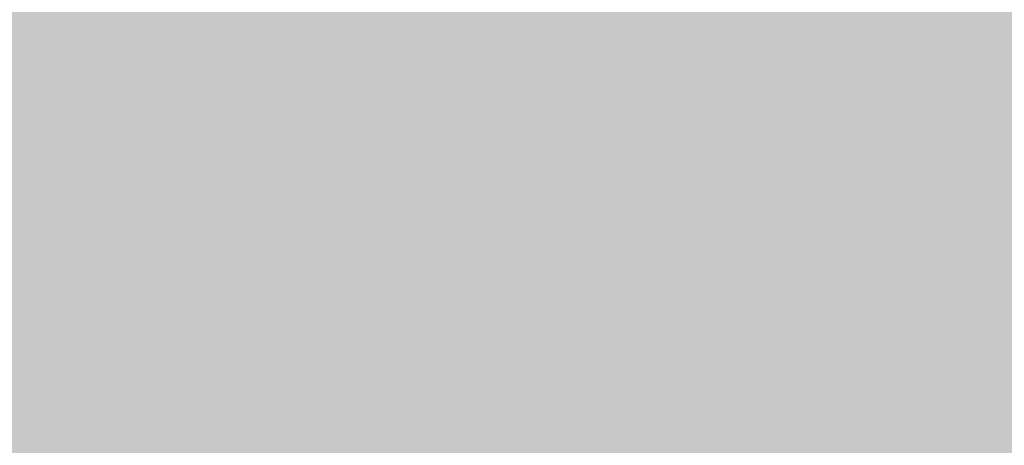
# Model space of a CAD drawing. Units: millimetres. Extents: x -22994 to 29398, y -19990 to 20176.
# Tile 74 of 135: x 226.355 to 227.437, y 83.796 to 84.264. Entities that reach past the tile are written whole.
import ezdxf
from ezdxf import colors
from ezdxf.entities.mleader import LeaderData, LeaderLine
from ezdxf.math import Vec2, Vec3

# ---------------------------------------------------------------- set-up
doc = ezdxf.new("R2010")
doc.units = ezdxf.units.MM
doc.header["$MEASUREMENT"] = 0
for name, color, linetype, lineweight in [('M-ANNO-TEXT', 7, 'Continuous', 25), ('M-DIMS', 2, 'Continuous', 18), ('M-EQPM-PATT', 7, 'Continuous', 18)]:
    doc.layers.add(name, color=color, linetype=linetype, lineweight=lineweight)
doc.styles.get("Standard").update_dxf_attribs({"font": 'arial.ttf'})
doc.dimstyles.get("Standard").update_dxf_attribs({"dimtxt": 0.18, "dimasz": 10000, "dimexe": 0.18, "dimexo": 0.0625, "dimgap": 0.09, "dimtad": 0, "dimtih": 1, "dimtoh": 1, "dimdec": 0, "dimzin": 0, "dimdsep": 46, "dimtxsty": 'Standard', "dimcen": 0.09, "dimadec": 0, "dimazin": 0, "dimtfac": 1, "dimtdec": 0, "dimtofl": 0, "dimtmove": 0, "dimatfit": 3, "dimfxl": 1, "dimtolj": 1, "dimtzin": 0, "dimlwd": 30, "dimarcsym": 0})

# ---------------------------------------------------------------- blocks, each defined once
blk = doc.blocks.new('*D2')
at = {"layer": 'Defpoints', "color": 0, "transparency": 16777216}
for p in [(6.6773, 10.2713), (290.852, 10.2713), (290.852, -5.0787)]:
    blk.add_point(p, dxfattribs=at)
at = {"layer": 'M-DIMS', "color": 0, "lineweight": -2, "transparency": 16777216}
for p, q in [((6.6773, 10.2088), (6.6773, -5.2587)), ((290.852, 10.2088), (290.852, -5.2587))]:
    blk.add_line(p, q, dxfattribs=at)
at = {"layer": 'M-DIMS', "color": 0, "lineweight": 30, "transparency": 16777216}
for p, q in [((-9993.3227, -5.0787), (-19993.3227, -5.0787)), ((10290.852, -5.0787), (20290.852, -5.0787))]:
    blk.add_line(p, q, dxfattribs=at)
at = {"layer": 'M-DIMS', "color": 0, "transparency": 16777216}
for points in [[(-9993.3227, 1661.5879), (-9993.3227, -1671.7454), (6.6773, -5.0787)], [(10290.852, 1661.5879), (10290.852, -1671.7454), (290.852, -5.0787)]]:
    blk.add_solid(points, dxfattribs=at)
at = {"layer": 'M-DIMS', "color": 0, "transparency": 16777216, "insert": (148.7647, -5.0787), "char_height": 0.18, "attachment_point": 5}
blk.add_mtext('\\A1;284.2', dxfattribs=at)
blk = doc.blocks.new('*D3')
at = {"layer": 'Defpoints', "color": 0, "transparency": 16777216}
for p in [(110.2647, 204.1654), (110.2647, 176.3662), (95.8327, 127.967)]:
    blk.add_point(p, dxfattribs=at)
at = {"layer": 'M-DIMS', "color": 0, "lineweight": -2, "transparency": 16777216}
for p, q in [((95.8327, 128.0295), (95.8327, 204.3454)), ((110.2647, 176.4287), (110.2647, 204.3454))]:
    blk.add_line(p, q, dxfattribs=at)
at = {"layer": 'M-DIMS', "color": 0, "lineweight": 30, "transparency": 16777216}
for p, q in [((-9904.1673, 204.1654), (-19904.1673, 204.1654)), ((10110.2647, 204.1654), (20110.2647, 204.1654))]:
    blk.add_line(p, q, dxfattribs=at)
at = {"layer": 'M-DIMS', "color": 0, "transparency": 16777216}
for points in [[(-9904.1673, 1870.8321), (-9904.1673, -1462.5013), (95.8327, 204.1654)], [(10110.2647, 1870.8321), (10110.2647, -1462.5013), (110.2647, 204.1654)]]:
    blk.add_solid(points, dxfattribs=at)
at = {"layer": 'M-DIMS', "color": 0, "transparency": 16777216, "insert": (103.0487, 204.1654), "char_height": 0.18, "attachment_point": 5}
blk.add_mtext('\\A1;14.432', dxfattribs=at)
blk = doc.blocks.new('*D4')
at = {"layer": 'Defpoints', "color": 0, "transparency": 16777216}
for p in [(116.2647, 204.1654), (110.2647, 176.3662), (116.2647, 176.3662)]:
    blk.add_point(p, dxfattribs=at)
at = {"layer": 'M-DIMS', "color": 0, "lineweight": -2, "transparency": 16777216}
for p, q in [((110.2647, 176.4287), (110.2647, 204.3454)), ((116.2647, 176.4287), (116.2647, 204.3454))]:
    blk.add_line(p, q, dxfattribs=at)
at = {"layer": 'M-DIMS', "color": 0, "lineweight": 30, "transparency": 16777216}
for p, q in [((-9889.7353, 204.1654), (-19889.7353, 204.1654)), ((10116.2647, 204.1654), (20116.2647, 204.1654))]:
    blk.add_line(p, q, dxfattribs=at)
at = {"layer": 'M-DIMS', "color": 0, "transparency": 16777216}
for points in [[(-9889.7353, 1870.8321), (-9889.7353, -1462.5013), (110.2647, 204.1654)], [(10116.2647, 1870.8321), (10116.2647, -1462.5013), (116.2647, 204.1654)]]:
    blk.add_solid(points, dxfattribs=at)
at = {"layer": 'M-DIMS', "color": 0, "transparency": 16777216, "insert": (113.2647, 204.1654), "char_height": 0.18, "attachment_point": 5}
blk.add_mtext('\\A1;6', dxfattribs=at)
blk = doc.blocks.new('*D5')
at = {"layer": 'Defpoints', "color": 0, "transparency": 16777216}
for p in [(181.2647, 204.1654), (116.2647, 176.3662), (181.2647, 176.3662)]:
    blk.add_point(p, dxfattribs=at)
at = {"layer": 'M-DIMS', "color": 0, "lineweight": -2, "transparency": 16777216}
for p, q in [((116.2647, 176.4287), (116.2647, 204.3454)), ((181.2647, 176.4287), (181.2647, 204.3454))]:
    blk.add_line(p, q, dxfattribs=at)
at = {"layer": 'M-DIMS', "color": 0, "lineweight": 30, "transparency": 16777216}
for p, q in [((-9883.7353, 204.1654), (-19883.7353, 204.1654)), ((10181.2647, 204.1654), (20181.2647, 204.1654))]:
    blk.add_line(p, q, dxfattribs=at)
at = {"layer": 'M-DIMS', "color": 0, "transparency": 16777216}
for points in [[(-9883.7353, 1870.8321), (-9883.7353, -1462.5013), (116.2647, 204.1654)], [(10181.2647, 1870.8321), (10181.2647, -1462.5013), (181.2647, 204.1654)]]:
    blk.add_solid(points, dxfattribs=at)
at = {"layer": 'M-DIMS', "color": 0, "transparency": 16777216, "insert": (148.7647, 204.1654), "char_height": 0.18, "attachment_point": 5}
blk.add_mtext('\\A1;65', dxfattribs=at)
blk = doc.blocks.new('*D6')
at = {"layer": 'Defpoints', "color": 0, "transparency": 16777216}
for p in [(187.2647, 204.1654), (181.2647, 176.3662), (187.2647, 176.3662)]:
    blk.add_point(p, dxfattribs=at)
at = {"layer": 'M-DIMS', "color": 0, "lineweight": -2, "transparency": 16777216}
for p, q in [((181.2647, 176.4287), (181.2647, 204.3454)), ((187.2647, 176.4287), (187.2647, 204.3454))]:
    blk.add_line(p, q, dxfattribs=at)
at = {"layer": 'M-DIMS', "color": 0, "lineweight": 30, "transparency": 16777216}
for p, q in [((-9818.7353, 204.1654), (-19818.7353, 204.1654)), ((10187.2647, 204.1654), (20187.2647, 204.1654))]:
    blk.add_line(p, q, dxfattribs=at)
at = {"layer": 'M-DIMS', "color": 0, "transparency": 16777216}
for points in [[(-9818.7353, 1870.8321), (-9818.7353, -1462.5013), (181.2647, 204.1654)], [(10187.2647, 1870.8321), (10187.2647, -1462.5013), (187.2647, 204.1654)]]:
    blk.add_solid(points, dxfattribs=at)
at = {"layer": 'M-DIMS', "color": 0, "transparency": 16777216, "insert": (184.2647, 204.1654), "char_height": 0.18, "attachment_point": 5}
blk.add_mtext('\\A1;6', dxfattribs=at)
blk = doc.blocks.new('*D7')
at = {"layer": 'Defpoints', "color": 0, "transparency": 16777216}
for p in [(201.6967, 204.1654), (187.2647, 176.3662), (201.6967, 127.967)]:
    blk.add_point(p, dxfattribs=at)
at = {"layer": 'M-DIMS', "color": 0, "lineweight": -2, "transparency": 16777216}
for p, q in [((187.2647, 176.4287), (187.2647, 204.3454)), ((201.6967, 128.0295), (201.6967, 204.3454))]:
    blk.add_line(p, q, dxfattribs=at)
at = {"layer": 'M-DIMS', "color": 0, "lineweight": 30, "transparency": 16777216}
for p, q in [((-9812.7353, 204.1654), (-19812.7353, 204.1654)), ((10201.6967, 204.1654), (20201.6967, 204.1654))]:
    blk.add_line(p, q, dxfattribs=at)
at = {"layer": 'M-DIMS', "color": 0, "transparency": 16777216}
for points in [[(-9812.7353, 1870.8321), (-9812.7353, -1462.5013), (187.2647, 204.1654)], [(10201.6967, 1870.8321), (10201.6967, -1462.5013), (201.6967, 204.1654)]]:
    blk.add_solid(points, dxfattribs=at)
at = {"layer": 'M-DIMS', "color": 0, "transparency": 16777216, "insert": (194.4807, 204.1654), "char_height": 0.18, "attachment_point": 5}
blk.add_mtext('\\A1;14.432', dxfattribs=at)
blk = doc.blocks.new('*D8')
at = {"layer": 'Defpoints', "color": 0, "transparency": 16777216}
for p in [(227.6485, 204.1654), (227.6485, 146.7296), (201.6967, 127.967)]:
    blk.add_point(p, dxfattribs=at)
at = {"layer": 'M-DIMS', "color": 0, "lineweight": -2, "transparency": 16777216}
for p, q in [((201.6967, 128.0295), (201.6967, 204.3454)), ((227.6485, 146.7921), (227.6485, 204.3454))]:
    blk.add_line(p, q, dxfattribs=at)
at = {"layer": 'M-DIMS', "color": 0, "lineweight": 30, "transparency": 16777216}
for p, q in [((-9798.3033, 204.1654), (-19798.3033, 204.1654)), ((10227.6485, 204.1654), (20227.6485, 204.1654))]:
    blk.add_line(p, q, dxfattribs=at)
at = {"layer": 'M-DIMS', "color": 0, "transparency": 16777216}
for points in [[(-9798.3033, 1870.8321), (-9798.3033, -1462.5013), (201.6967, 204.1654)], [(10227.6485, 1870.8321), (10227.6485, -1462.5013), (227.6485, 204.1654)]]:
    blk.add_solid(points, dxfattribs=at)
at = {"layer": 'M-DIMS', "color": 0, "transparency": 16777216, "insert": (214.6726, 204.1654), "char_height": 0.18, "attachment_point": 5}
blk.add_mtext('\\A1;25.95', dxfattribs=at)
blk = doc.blocks.new('*D9')
at = {"layer": 'Defpoints', "color": 0, "transparency": 16777216}
for p in [(187.2647, 176.3662), (306.202, 176.3662), (290.852, 10.2713)]:
    blk.add_point(p, dxfattribs=at)
at = {"layer": 'M-DIMS', "color": 0, "lineweight": 30, "transparency": 16777216}
for p, q in [((306.202, 10176.3662), (306.202, 20176.3662)), ((306.202, -9989.7287), (306.202, -19989.7287))]:
    blk.add_line(p, q, dxfattribs=at)
at = {"layer": 'M-DIMS', "color": 0, "lineweight": -2, "transparency": 16777216}
for p, q in [((187.3272, 176.3662), (306.382, 176.3662)), ((290.9145, 10.2713), (306.382, 10.2713))]:
    blk.add_line(p, q, dxfattribs=at)
at = {"layer": 'M-DIMS', "color": 0, "transparency": 16777216}
for points in [[(-1360.4646, 10176.3662), (1972.8687, 10176.3662), (306.202, 176.3662)], [(-1360.4646, -9989.7287), (1972.8687, -9989.7287), (306.202, 10.2713)]]:
    blk.add_solid(points, dxfattribs=at)
at = {"layer": 'M-DIMS', "color": 0, "transparency": 16777216, "insert": (306.202, 93.3187), "char_height": 0.18, "attachment_point": 5}
blk.add_mtext('\\A1;166.1', dxfattribs=at)
blk = doc.blocks.new('*D10')
at = {"layer": 'Defpoints', "color": 0, "transparency": 16777216}
for p in [(125.6498, 136.0713), (133.3459, 136.0713), (133.3459, -5.0787)]:
    blk.add_point(p, dxfattribs=at)
at = {"layer": 'M-DIMS', "color": 0, "lineweight": -2, "transparency": 16777216}
for p, q in [((125.6498, 136.0088), (125.6498, -5.2587)), ((133.3459, 136.0088), (133.3459, -5.2587))]:
    blk.add_line(p, q, dxfattribs=at)
at = {"layer": 'M-DIMS', "color": 0, "lineweight": 30, "transparency": 16777216}
for p, q in [((-9874.3502, -5.0787), (-19874.3502, -5.0787)), ((10133.3459, -5.0787), (20133.3459, -5.0787))]:
    blk.add_line(p, q, dxfattribs=at)
at = {"layer": 'M-DIMS', "color": 0, "transparency": 16777216}
for points in [[(-9874.3502, 1661.5879), (-9874.3502, -1671.7454), (125.6498, -5.0787)], [(10133.3459, 1661.5879), (10133.3459, -1671.7454), (133.3459, -5.0787)]]:
    blk.add_solid(points, dxfattribs=at)
at = {"layer": 'M-DIMS', "color": 0, "transparency": 16777216, "insert": (129.4978, -5.0787), "char_height": 0.18, "attachment_point": 5}
blk.add_mtext('\\A1;7.696', dxfattribs=at)
blk = doc.blocks.new('*D11')
at = {"layer": 'Defpoints', "color": 0, "transparency": 16777216}
for p in [(133.3459, 136.0713), (135.6498, 136.0713), (135.6498, -5.0787)]:
    blk.add_point(p, dxfattribs=at)
at = {"layer": 'M-DIMS', "color": 0, "lineweight": -2, "transparency": 16777216}
for p, q in [((133.3459, 136.0088), (133.3459, -5.2587)), ((135.6498, 136.0088), (135.6498, -5.2587))]:
    blk.add_line(p, q, dxfattribs=at)
at = {"layer": 'M-DIMS', "color": 0, "lineweight": 30, "transparency": 16777216}
for p, q in [((-9866.6541, -5.0787), (-19866.6541, -5.0787)), ((10135.6498, -5.0787), (20135.6498, -5.0787))]:
    blk.add_line(p, q, dxfattribs=at)
at = {"layer": 'M-DIMS', "color": 0, "transparency": 16777216}
for points in [[(-9866.6541, 1661.5879), (-9866.6541, -1671.7454), (133.3459, -5.0787)], [(10135.6498, 1661.5879), (10135.6498, -1671.7454), (135.6498, -5.0787)]]:
    blk.add_solid(points, dxfattribs=at)
at = {"layer": 'M-DIMS', "color": 0, "transparency": 16777216, "insert": (134.4978, -5.0787), "char_height": 0.18, "attachment_point": 5}
blk.add_mtext('\\A1;2.304', dxfattribs=at)
blk = doc.blocks.new('*D12')
at = {"layer": 'Defpoints', "color": 0, "transparency": 16777216}
for p in [(135.6498, 136.0713), (145.6498, 136.0713), (145.6498, -5.0787)]:
    blk.add_point(p, dxfattribs=at)
at = {"layer": 'M-DIMS', "color": 0, "lineweight": -2, "transparency": 16777216}
for p, q in [((135.6498, 136.0088), (135.6498, -5.2587)), ((145.6498, 136.0088), (145.6498, -5.2587))]:
    blk.add_line(p, q, dxfattribs=at)
at = {"layer": 'M-DIMS', "color": 0, "lineweight": 30, "transparency": 16777216}
for p, q in [((-9864.3502, -5.0787), (-19864.3502, -5.0787)), ((10145.6498, -5.0787), (20145.6498, -5.0787))]:
    blk.add_line(p, q, dxfattribs=at)
at = {"layer": 'M-DIMS', "color": 0, "transparency": 16777216}
for points in [[(-9864.3502, 1661.5879), (-9864.3502, -1671.7454), (135.6498, -5.0787)], [(10145.6498, 1661.5879), (10145.6498, -1671.7454), (145.6498, -5.0787)]]:
    blk.add_solid(points, dxfattribs=at)
at = {"layer": 'M-DIMS', "color": 0, "transparency": 16777216, "insert": (140.6498, -5.0787), "char_height": 0.18, "attachment_point": 5}
blk.add_mtext('\\A1;10', dxfattribs=at)
blk = doc.blocks.new('*D13')
at = {"layer": 'Defpoints', "color": 0, "transparency": 16777216}
for p in [(145.6498, 136.0713), (155.6498, 136.0713), (155.6498, -5.0787)]:
    blk.add_point(p, dxfattribs=at)
at = {"layer": 'M-DIMS', "color": 0, "lineweight": -2, "transparency": 16777216}
for p, q in [((145.6498, 136.0088), (145.6498, -5.2587)), ((155.6498, 136.0088), (155.6498, -5.2587))]:
    blk.add_line(p, q, dxfattribs=at)
at = {"layer": 'M-DIMS', "color": 0, "lineweight": 30, "transparency": 16777216}
for p, q in [((-9854.3502, -5.0787), (-19854.3502, -5.0787)), ((10155.6498, -5.0787), (20155.6498, -5.0787))]:
    blk.add_line(p, q, dxfattribs=at)
at = {"layer": 'M-DIMS', "color": 0, "transparency": 16777216}
for points in [[(-9854.3502, 1661.5879), (-9854.3502, -1671.7454), (145.6498, -5.0787)], [(10155.6498, 1661.5879), (10155.6498, -1671.7454), (155.6498, -5.0787)]]:
    blk.add_solid(points, dxfattribs=at)
at = {"layer": 'M-DIMS', "color": 0, "transparency": 16777216, "insert": (150.6498, -5.0787), "char_height": 0.18, "attachment_point": 5}
blk.add_mtext('\\A1;10', dxfattribs=at)
blk = doc.blocks.new('*D14')
at = {"layer": 'Defpoints', "color": 0, "transparency": 16777216}
for p in [(155.6498, 136.0713), (165.6498, 136.0713), (165.6498, -5.0787)]:
    blk.add_point(p, dxfattribs=at)
at = {"layer": 'M-DIMS', "color": 0, "lineweight": -2, "transparency": 16777216}
for p, q in [((155.6498, 136.0088), (155.6498, -5.2587)), ((165.6498, 136.0088), (165.6498, -5.2587))]:
    blk.add_line(p, q, dxfattribs=at)
at = {"layer": 'M-DIMS', "color": 0, "lineweight": 30, "transparency": 16777216}
for p, q in [((-9844.3502, -5.0787), (-19844.3502, -5.0787)), ((10165.6498, -5.0787), (20165.6498, -5.0787))]:
    blk.add_line(p, q, dxfattribs=at)
at = {"layer": 'M-DIMS', "color": 0, "transparency": 16777216}
for points in [[(-9844.3502, 1661.5879), (-9844.3502, -1671.7454), (155.6498, -5.0787)], [(10165.6498, 1661.5879), (10165.6498, -1671.7454), (165.6498, -5.0787)]]:
    blk.add_solid(points, dxfattribs=at)
at = {"layer": 'M-DIMS', "color": 0, "transparency": 16777216, "insert": (160.6498, -5.0787), "char_height": 0.18, "attachment_point": 5}
blk.add_mtext('\\A1;10', dxfattribs=at)
blk = doc.blocks.new('*D15')
at = {"layer": 'Defpoints', "color": 0, "transparency": 16777216}
for p in [(173.3459, 154.788), (173.3459, 136.0713), (306.202, 136.0713)]:
    blk.add_point(p, dxfattribs=at)
at = {"layer": 'M-DIMS', "color": 0, "lineweight": 30, "transparency": 16777216}
for p, q in [((306.202, 10154.788), (306.202, 20154.788)), ((306.202, -9863.9287), (306.202, -19863.9287))]:
    blk.add_line(p, q, dxfattribs=at)
at = {"layer": 'M-DIMS', "color": 0, "lineweight": -2, "transparency": 16777216}
for p, q in [((173.4084, 154.788), (306.382, 154.788)), ((173.4084, 136.0713), (306.382, 136.0713))]:
    blk.add_line(p, q, dxfattribs=at)
at = {"layer": 'M-DIMS', "color": 0, "transparency": 16777216}
for points in [[(-1360.4646, 10154.788), (1972.8687, 10154.788), (306.202, 154.788)], [(-1360.4646, -9863.9287), (1972.8687, -9863.9287), (306.202, 136.0713)]]:
    blk.add_solid(points, dxfattribs=at)
at = {"layer": 'M-DIMS', "color": 0, "transparency": 16777216, "insert": (306.202, 145.4297), "char_height": 0.18, "attachment_point": 5}
blk.add_mtext('\\A1;18.717', dxfattribs=at)
blk = doc.blocks.new('*D16')
at = {"layer": 'Defpoints', "color": 0, "transparency": 16777216}
for p in [(120.1702, 204.1654), (110.4658, 48.0349), (120.1702, 48.0349)]:
    blk.add_point(p, dxfattribs=at)
at = {"layer": 'M-DIMS', "color": 0, "lineweight": -2, "transparency": 16777216}
for p, q in [((110.4658, 48.0974), (110.4658, 204.3454)), ((120.1702, 48.0974), (120.1702, 204.3454))]:
    blk.add_line(p, q, dxfattribs=at)
at = {"layer": 'M-DIMS', "color": 0, "lineweight": 30, "transparency": 16777216}
for p, q in [((-9889.5342, 204.1654), (-19889.5342, 204.1654)), ((10120.1702, 204.1654), (20120.1702, 204.1654))]:
    blk.add_line(p, q, dxfattribs=at)
at = {"layer": 'M-DIMS', "color": 0, "transparency": 16777216}
for points in [[(-9889.5342, 1870.8321), (-9889.5342, -1462.5013), (110.4658, 204.1654)], [(10120.1702, 1870.8321), (10120.1702, -1462.5013), (120.1702, 204.1654)]]:
    blk.add_solid(points, dxfattribs=at)
at = {"layer": 'M-DIMS', "color": 0, "transparency": 16777216, "insert": (115.318, 204.1654), "char_height": 0.18, "attachment_point": 5}
blk.add_mtext('\\A1;9.704', dxfattribs=at)
blk = doc.blocks.new('*D17')
at = {"layer": 'Defpoints', "color": 0, "transparency": 16777216}
for p in [(126.1702, 204.1654), (120.1702, 48.0349), (126.1702, 48.0349)]:
    blk.add_point(p, dxfattribs=at)
at = {"layer": 'M-DIMS', "color": 0, "lineweight": -2, "transparency": 16777216}
for p, q in [((120.1702, 48.0974), (120.1702, 204.3454)), ((126.1702, 48.0974), (126.1702, 204.3454))]:
    blk.add_line(p, q, dxfattribs=at)
at = {"layer": 'M-DIMS', "color": 0, "lineweight": 30, "transparency": 16777216}
for p, q in [((-9879.8298, 204.1654), (-19879.8298, 204.1654)), ((10126.1702, 204.1654), (20126.1702, 204.1654))]:
    blk.add_line(p, q, dxfattribs=at)
at = {"layer": 'M-DIMS', "color": 0, "transparency": 16777216}
for points in [[(-9879.8298, 1870.8321), (-9879.8298, -1462.5013), (120.1702, 204.1654)], [(10126.1702, 1870.8321), (10126.1702, -1462.5013), (126.1702, 204.1654)]]:
    blk.add_solid(points, dxfattribs=at)
at = {"layer": 'M-DIMS', "color": 0, "transparency": 16777216, "insert": (123.1702, 204.1654), "char_height": 0.18, "attachment_point": 5}
blk.add_mtext('\\A1;6', dxfattribs=at)
blk = doc.blocks.new('*D18')
at = {"layer": 'Defpoints', "color": 0, "transparency": 16777216}
for p in [(132.1702, 204.1654), (126.1702, 48.0349), (132.1702, 48.0349)]:
    blk.add_point(p, dxfattribs=at)
at = {"layer": 'M-DIMS', "color": 0, "lineweight": -2, "transparency": 16777216}
for p, q in [((126.1702, 48.0974), (126.1702, 204.3454)), ((132.1702, 48.0974), (132.1702, 204.3454))]:
    blk.add_line(p, q, dxfattribs=at)
at = {"layer": 'M-DIMS', "color": 0, "lineweight": 30, "transparency": 16777216}
for p, q in [((-9873.8298, 204.1654), (-19873.8298, 204.1654)), ((10132.1702, 204.1654), (20132.1702, 204.1654))]:
    blk.add_line(p, q, dxfattribs=at)
at = {"layer": 'M-DIMS', "color": 0, "transparency": 16777216}
for points in [[(-9873.8298, 1870.8321), (-9873.8298, -1462.5013), (126.1702, 204.1654)], [(10132.1702, 1870.8321), (10132.1702, -1462.5013), (132.1702, 204.1654)]]:
    blk.add_solid(points, dxfattribs=at)
at = {"layer": 'M-DIMS', "color": 0, "transparency": 16777216, "insert": (129.1702, 204.1654), "char_height": 0.18, "attachment_point": 5}
blk.add_mtext('\\A1;6', dxfattribs=at)
blk = doc.blocks.new('*D19')
at = {"layer": 'Defpoints', "color": 0, "transparency": 16777216}
for p in [(138.1702, 204.1654), (132.1702, 48.0349), (138.1702, 48.0349)]:
    blk.add_point(p, dxfattribs=at)
at = {"layer": 'M-DIMS', "color": 0, "lineweight": -2, "transparency": 16777216}
for p, q in [((132.1702, 48.0974), (132.1702, 204.3454)), ((138.1702, 48.0974), (138.1702, 204.3454))]:
    blk.add_line(p, q, dxfattribs=at)
at = {"layer": 'M-DIMS', "color": 0, "lineweight": 30, "transparency": 16777216}
for p, q in [((-9867.8298, 204.1654), (-19867.8298, 204.1654)), ((10138.1702, 204.1654), (20138.1702, 204.1654))]:
    blk.add_line(p, q, dxfattribs=at)
at = {"layer": 'M-DIMS', "color": 0, "transparency": 16777216}
for points in [[(-9867.8298, 1870.8321), (-9867.8298, -1462.5013), (132.1702, 204.1654)], [(10138.1702, 1870.8321), (10138.1702, -1462.5013), (138.1702, 204.1654)]]:
    blk.add_solid(points, dxfattribs=at)
at = {"layer": 'M-DIMS', "color": 0, "transparency": 16777216, "insert": (135.1702, 204.1654), "char_height": 0.18, "attachment_point": 5}
blk.add_mtext('\\A1;6', dxfattribs=at)
blk = doc.blocks.new('*D20')
at = {"layer": 'Defpoints', "color": 0, "transparency": 16777216}
for p in [(144.1702, 204.1654), (138.1702, 48.0349), (144.1702, 48.0349)]:
    blk.add_point(p, dxfattribs=at)
at = {"layer": 'M-DIMS', "color": 0, "lineweight": -2, "transparency": 16777216}
for p, q in [((138.1702, 48.0974), (138.1702, 204.3454)), ((144.1702, 48.0974), (144.1702, 204.3454))]:
    blk.add_line(p, q, dxfattribs=at)
at = {"layer": 'M-DIMS', "color": 0, "lineweight": 30, "transparency": 16777216}
for p, q in [((-9861.8298, 204.1654), (-19861.8298, 204.1654)), ((10144.1702, 204.1654), (20144.1702, 204.1654))]:
    blk.add_line(p, q, dxfattribs=at)
at = {"layer": 'M-DIMS', "color": 0, "transparency": 16777216}
for points in [[(-9861.8298, 1870.8321), (-9861.8298, -1462.5013), (138.1702, 204.1654)], [(10144.1702, 1870.8321), (10144.1702, -1462.5013), (144.1702, 204.1654)]]:
    blk.add_solid(points, dxfattribs=at)
at = {"layer": 'M-DIMS', "color": 0, "transparency": 16777216, "insert": (141.1702, 204.1654), "char_height": 0.18, "attachment_point": 5}
blk.add_mtext('\\A1;6', dxfattribs=at)
blk = doc.blocks.new('*D21')
at = {"layer": 'Defpoints', "color": 0, "transparency": 16777216}
for p in [(149.1157, 204.1654), (144.1702, 48.0349), (149.1157, 48.0349)]:
    blk.add_point(p, dxfattribs=at)
at = {"layer": 'M-DIMS', "color": 0, "lineweight": -2, "transparency": 16777216}
for p, q in [((144.1702, 48.0974), (144.1702, 204.3454)), ((149.1157, 48.0974), (149.1157, 204.3454))]:
    blk.add_line(p, q, dxfattribs=at)
at = {"layer": 'M-DIMS', "color": 0, "lineweight": 30, "transparency": 16777216}
for p, q in [((-9855.8298, 204.1654), (-19855.8298, 204.1654)), ((10149.1157, 204.1654), (20149.1157, 204.1654))]:
    blk.add_line(p, q, dxfattribs=at)
at = {"layer": 'M-DIMS', "color": 0, "transparency": 16777216}
for points in [[(-9855.8298, 1870.8321), (-9855.8298, -1462.5013), (144.1702, 204.1654)], [(10149.1157, 1870.8321), (10149.1157, -1462.5013), (149.1157, 204.1654)]]:
    blk.add_solid(points, dxfattribs=at)
at = {"layer": 'M-DIMS', "color": 0, "transparency": 16777216, "insert": (146.6429, 204.1654), "char_height": 0.18, "attachment_point": 5}
blk.add_mtext('\\A1;4.945', dxfattribs=at)
blk = doc.blocks.new('*D22')
at = {"layer": 'Defpoints', "color": 0, "transparency": 16777216}
for p in [(149.1157, 30.9895), (155.1157, 30.9895), (155.1157, -5.0787)]:
    blk.add_point(p, dxfattribs=at)
at = {"layer": 'M-DIMS', "color": 0, "lineweight": -2, "transparency": 16777216}
for p, q in [((149.1157, 30.927), (149.1157, -5.2587)), ((155.1157, 30.927), (155.1157, -5.2587))]:
    blk.add_line(p, q, dxfattribs=at)
at = {"layer": 'M-DIMS', "color": 0, "lineweight": 30, "transparency": 16777216}
for p, q in [((-9850.8843, -5.0787), (-19850.8843, -5.0787)), ((10155.1157, -5.0787), (20155.1157, -5.0787))]:
    blk.add_line(p, q, dxfattribs=at)
at = {"layer": 'M-DIMS', "color": 0, "transparency": 16777216}
for points in [[(-9850.8843, 1661.5879), (-9850.8843, -1671.7454), (149.1157, -5.0787)], [(10155.1157, 1661.5879), (10155.1157, -1671.7454), (155.1157, -5.0787)]]:
    blk.add_solid(points, dxfattribs=at)
at = {"layer": 'M-DIMS', "color": 0, "transparency": 16777216, "insert": (152.1157, -5.0787), "char_height": 0.18, "attachment_point": 5}
blk.add_mtext('\\A1;6', dxfattribs=at)
blk = doc.blocks.new('*D23')
at = {"layer": 'Defpoints', "color": 0, "transparency": 16777216}
for p in [(155.1157, 30.9895), (161.1157, 30.9895), (161.1157, -5.0787)]:
    blk.add_point(p, dxfattribs=at)
at = {"layer": 'M-DIMS', "color": 0, "lineweight": -2, "transparency": 16777216}
for p, q in [((155.1157, 30.927), (155.1157, -5.2587)), ((161.1157, 30.927), (161.1157, -5.2587))]:
    blk.add_line(p, q, dxfattribs=at)
at = {"layer": 'M-DIMS', "color": 0, "lineweight": 30, "transparency": 16777216}
for p, q in [((-9844.8843, -5.0787), (-19844.8843, -5.0787)), ((10161.1157, -5.0787), (20161.1157, -5.0787))]:
    blk.add_line(p, q, dxfattribs=at)
at = {"layer": 'M-DIMS', "color": 0, "transparency": 16777216}
for points in [[(-9844.8843, 1661.5879), (-9844.8843, -1671.7454), (155.1157, -5.0787)], [(10161.1157, 1661.5879), (10161.1157, -1671.7454), (161.1157, -5.0787)]]:
    blk.add_solid(points, dxfattribs=at)
at = {"layer": 'M-DIMS', "color": 0, "transparency": 16777216, "insert": (158.1157, -5.0787), "char_height": 0.18, "attachment_point": 5}
blk.add_mtext('\\A1;6', dxfattribs=at)
blk = doc.blocks.new('*D24')
at = {"layer": 'Defpoints', "color": 0, "transparency": 16777216}
for p in [(161.1157, 30.9895), (166.4387, 30.9895), (166.4387, -5.0787)]:
    blk.add_point(p, dxfattribs=at)
at = {"layer": 'M-DIMS', "color": 0, "lineweight": -2, "transparency": 16777216}
for p, q in [((161.1157, 30.927), (161.1157, -5.2587)), ((166.4387, 30.927), (166.4387, -5.2587))]:
    blk.add_line(p, q, dxfattribs=at)
at = {"layer": 'M-DIMS', "color": 0, "lineweight": 30, "transparency": 16777216}
for p, q in [((-9838.8843, -5.0787), (-19838.8843, -5.0787)), ((10166.4387, -5.0787), (20166.4387, -5.0787))]:
    blk.add_line(p, q, dxfattribs=at)
at = {"layer": 'M-DIMS', "color": 0, "transparency": 16777216}
for points in [[(-9838.8843, 1661.5879), (-9838.8843, -1671.7454), (161.1157, -5.0787)], [(10166.4387, 1661.5879), (10166.4387, -1671.7454), (166.4387, -5.0787)]]:
    blk.add_solid(points, dxfattribs=at)
at = {"layer": 'M-DIMS', "color": 0, "transparency": 16777216, "insert": (163.7772, -5.0787), "char_height": 0.18, "attachment_point": 5}
blk.add_mtext('\\A1;5.323', dxfattribs=at)
blk = doc.blocks.new('*D25')
at = {"layer": 'Defpoints', "color": 0, "transparency": 16777216}
for p in [(166.4387, 30.9895), (172.4387, 30.9895), (172.4387, -5.0787)]:
    blk.add_point(p, dxfattribs=at)
at = {"layer": 'M-DIMS', "color": 0, "lineweight": -2, "transparency": 16777216}
for p, q in [((166.4387, 30.927), (166.4387, -5.2587)), ((172.4387, 30.927), (172.4387, -5.2587))]:
    blk.add_line(p, q, dxfattribs=at)
at = {"layer": 'M-DIMS', "color": 0, "lineweight": 30, "transparency": 16777216}
for p, q in [((-9833.5613, -5.0787), (-19833.5613, -5.0787)), ((10172.4387, -5.0787), (20172.4387, -5.0787))]:
    blk.add_line(p, q, dxfattribs=at)
at = {"layer": 'M-DIMS', "color": 0, "transparency": 16777216}
for points in [[(-9833.5613, 1661.5879), (-9833.5613, -1671.7454), (166.4387, -5.0787)], [(10172.4387, 1661.5879), (10172.4387, -1671.7454), (172.4387, -5.0787)]]:
    blk.add_solid(points, dxfattribs=at)
at = {"layer": 'M-DIMS', "color": 0, "transparency": 16777216, "insert": (169.4387, -5.0787), "char_height": 0.18, "attachment_point": 5}
blk.add_mtext('\\A1;6', dxfattribs=at)
blk = doc.blocks.new('*D26')
at = {"layer": 'Defpoints', "color": 0, "transparency": 16777216}
for p in [(172.4387, 30.9895), (178.4387, 30.9895), (178.4387, -5.0787)]:
    blk.add_point(p, dxfattribs=at)
at = {"layer": 'M-DIMS', "color": 0, "lineweight": -2, "transparency": 16777216}
for p, q in [((172.4387, 30.927), (172.4387, -5.2587)), ((178.4387, 30.927), (178.4387, -5.2587))]:
    blk.add_line(p, q, dxfattribs=at)
at = {"layer": 'M-DIMS', "color": 0, "lineweight": 30, "transparency": 16777216}
for p, q in [((-9827.5613, -5.0787), (-19827.5613, -5.0787)), ((10178.4387, -5.0787), (20178.4387, -5.0787))]:
    blk.add_line(p, q, dxfattribs=at)
at = {"layer": 'M-DIMS', "color": 0, "transparency": 16777216}
for points in [[(-9827.5613, 1661.5879), (-9827.5613, -1671.7454), (172.4387, -5.0787)], [(10178.4387, 1661.5879), (10178.4387, -1671.7454), (178.4387, -5.0787)]]:
    blk.add_solid(points, dxfattribs=at)
at = {"layer": 'M-DIMS', "color": 0, "transparency": 16777216, "insert": (175.4387, -5.0787), "char_height": 0.18, "attachment_point": 5}
blk.add_mtext('\\A1;6', dxfattribs=at)
blk = doc.blocks.new('*D27')
at = {"layer": 'Defpoints', "color": 0, "transparency": 16777216}
for p in [(178.4387, 30.9895), (188.1175, 30.9895), (188.1175, -5.0787)]:
    blk.add_point(p, dxfattribs=at)
at = {"layer": 'M-DIMS', "color": 0, "lineweight": -2, "transparency": 16777216}
for p, q in [((178.4387, 30.927), (178.4387, -5.2587)), ((188.1175, 30.927), (188.1175, -5.2587))]:
    blk.add_line(p, q, dxfattribs=at)
at = {"layer": 'M-DIMS', "color": 0, "lineweight": 30, "transparency": 16777216}
for p, q in [((-9821.5613, -5.0787), (-19821.5613, -5.0787)), ((10188.1175, -5.0787), (20188.1175, -5.0787))]:
    blk.add_line(p, q, dxfattribs=at)
at = {"layer": 'M-DIMS', "color": 0, "transparency": 16777216}
for points in [[(-9821.5613, 1661.5879), (-9821.5613, -1671.7454), (178.4387, -5.0787)], [(10188.1175, 1661.5879), (10188.1175, -1671.7454), (188.1175, -5.0787)]]:
    blk.add_solid(points, dxfattribs=at)
at = {"layer": 'M-DIMS', "color": 0, "transparency": 16777216, "insert": (183.2781, -5.0787), "char_height": 0.18, "attachment_point": 5}
blk.add_mtext('\\A1;9.679', dxfattribs=at)
blk = doc.blocks.new('*D28')
at = {"layer": 'Defpoints', "color": 0, "transparency": 16777216}
for p in [(188.1175, 48.0349), (306.202, 48.0349), (188.1175, 30.9895)]:
    blk.add_point(p, dxfattribs=at)
at = {"layer": 'M-DIMS', "color": 0, "lineweight": 30, "transparency": 16777216}
for p, q in [((306.202, 10048.0349), (306.202, 20048.0349)), ((306.202, -9969.0105), (306.202, -19969.0105))]:
    blk.add_line(p, q, dxfattribs=at)
at = {"layer": 'M-DIMS', "color": 0, "lineweight": -2, "transparency": 16777216}
for p, q in [((188.18, 48.0349), (306.382, 48.0349)), ((188.18, 30.9895), (306.382, 30.9895))]:
    blk.add_line(p, q, dxfattribs=at)
at = {"layer": 'M-DIMS', "color": 0, "transparency": 16777216}
for points in [[(-1360.4646, 10048.0349), (1972.8687, 10048.0349), (306.202, 48.0349)], [(-1360.4646, -9969.0105), (1972.8687, -9969.0105), (306.202, 30.9895)]]:
    blk.add_solid(points, dxfattribs=at)
at = {"layer": 'M-DIMS', "color": 0, "transparency": 16777216, "insert": (306.202, 39.5122), "char_height": 0.18, "attachment_point": 5}
blk.add_mtext('\\A1;17.045', dxfattribs=at)
blk = doc.blocks.new('*D29')
at = {"layer": 'Defpoints', "color": 0, "transparency": 16777216}
for p in [(36.8006, 80.045), (64.0296, 80.045)]:
    blk.add_point(p, dxfattribs=at)
at = {"layer": 'M-DIMS', "color": 0, "lineweight": -2, "transparency": 16777216}
for p, q in [((50.4151, 79.955), (50.4151, 80.135)), ((50.3251, 80.045), (50.5051, 80.045))]:
    blk.add_line(p, q, dxfattribs=at)
at = {"layer": 'M-DIMS', "color": 0, "lineweight": 30, "transparency": 16777216}
blk.add_line((20064.0296, 80.0303), (10064.0296, 80.0377), dxfattribs=at)
at = {"layer": 'M-DIMS', "color": 0, "transparency": 16777216}
blk.add_solid([(10064.0309, 1746.7043), (10064.0284, -1586.629), (64.0296, 80.045)], dxfattribs=at)
at = {"layer": 'M-DIMS', "color": 0, "transparency": 16777216, "insert": (20064.5213, 80.0303), "char_height": 0.18, "attachment_point": 5}
blk.add_mtext('\\A1;∅27.23', dxfattribs=at)
blk = doc.blocks.new('*D30')
at = {"layer": 'Defpoints', "color": 0, "transparency": 16777216}
for p in [(216.3148, 146.7291), (238.9821, 146.73)]:
    blk.add_point(p, dxfattribs=at)
at = {"layer": 'M-DIMS', "color": 0, "lineweight": 30, "transparency": 16777216}
blk.add_line((20238.9821, 147.4959), (10238.9821, 147.1129), dxfattribs=at)
at = {"layer": 'M-DIMS', "color": 0, "lineweight": -2, "transparency": 16777216}
for p, q in [((227.6485, 146.6396), (227.6485, 146.8196)), ((227.5585, 146.7296), (227.7385, 146.7296))]:
    blk.add_line(p, q, dxfattribs=at)
at = {"layer": 'M-DIMS', "color": 0, "transparency": 16777216}
blk.add_solid([(10238.9183, 1813.7796), (10239.0459, -1519.5537), (238.9821, 146.73)], dxfattribs=at)
at = {"layer": 'M-DIMS', "color": 0, "transparency": 16777216, "insert": (20239.5436, 147.4959), "char_height": 0.18, "attachment_point": 5}
blk.add_mtext('\\A1;∅22.667', dxfattribs=at)
blk = doc.blocks.new('*D31')
at = {"layer": 'Defpoints', "color": 0, "transparency": 16777216}
for p in [(223.1641, 146.7291), (232.1328, 146.73)]:
    blk.add_point(p, dxfattribs=at)
at = {"layer": 'M-DIMS', "color": 0, "lineweight": 30, "transparency": 16777216}
blk.add_line((20232.1327, 148.6656), (10232.1328, 147.6978), dxfattribs=at)
at = {"layer": 'M-DIMS', "color": 0, "lineweight": -2, "transparency": 16777216}
for p, q in [((227.6485, 146.6396), (227.6485, 146.8196)), ((227.5585, 146.7296), (227.7385, 146.7296))]:
    blk.add_line(p, q, dxfattribs=at)
at = {"layer": 'M-DIMS', "color": 0, "transparency": 16777216}
blk.add_solid([(10231.9715, 1814.3645), (10232.2941, -1518.9688), (232.1328, 146.73)], dxfattribs=at)
at = {"layer": 'M-DIMS', "color": 0, "transparency": 16777216, "insert": (20232.6245, 148.6656), "char_height": 0.18, "attachment_point": 5}
blk.add_mtext('\\A1;∅8.969', dxfattribs=at)
blk = doc.blocks.new('*D36')
at = {"layer": 'Defpoints', "color": 0, "transparency": 16777216}
for p in [(46.39, 31.3035), (46.3875, 26.5934)]:
    blk.add_point(p, dxfattribs=at)
at = {"layer": 'M-DIMS', "color": 0, "lineweight": 30, "transparency": 16777216}
for p, q in [((57.1499, 20031.3006), (51.77, 10031.302)), ((10057.1499, 20031.3006), (57.1499, 20031.3006))]:
    blk.add_line(p, q, dxfattribs=at)
at = {"layer": 'M-DIMS', "color": 0, "lineweight": -2, "transparency": 16777216}
for p, q in [((46.3887, 28.8585), (46.3887, 29.0385)), ((46.2987, 28.9485), (46.4787, 28.9485))]:
    blk.add_line(p, q, dxfattribs=at)
at = {"layer": 'M-DIMS', "color": 0, "transparency": 16777216}
blk.add_solid([(-1614.8965, 10032.1987), (1718.4364, 10030.4054), (46.39, 31.3035)], dxfattribs=at)
at = {"layer": 'M-DIMS', "color": 0, "transparency": 16777216, "insert": (10057.5542, 20031.3006), "char_height": 0.18, "attachment_point": 5}
blk.add_mtext('\\A1;∅4.71', dxfattribs=at)

msp = doc.modelspace()

# ---------------------------------------------------------------- hatches: boundary and pattern name
at = {"layer": 'M-EQPM-PATT'}
h = msp.add_hatch(color=256, dxfattribs=at)
h.set_gradient(color1=(205, 32, 39), color2=(205, 32, 39), tint=1)
h.paths.add_polyline_path([(116.2647, 150.3662), (116.2647, 170.3662), (116.2647, 176.3662), (110.2647, 176.3662), (110.2647, 152.0276), (95.8327, 127.967), (95.8327, 16.6063), (201.6967, 16.6063), (201.6967, 127.967), (187.2647, 152.0276), (187.2647, 176.3662), (181.2647, 176.3662), (181.2647, 170.3662), (181.2647, 150.3662), (195.6967, 126.3055), (195.6967, 22.6063), (101.8327, 22.6063), (101.8327, 126.3055)])
h.paths.add_polyline_path([(185.2208, 88.6347), (101.8327, 88.6347), (101.8327, 87.6347), (182.8066, 87.6347), (178.7313, 83.5594), (195.6967, 83.5594), (195.6967, 84.5594), (181.1455, 84.5594)], flags=17)
h.paths.add_polyline_path([(95.8327, 88.6347), (60.9779, 88.6347, -0.022855), (61.7178, 87.6347), (95.8327, 87.6347)])
h.paths.add_polyline_path([(215.6212, 86.5189), (215.6212, 80.5999), (220.5095, 83.5594)])
h.paths.add_polyline_path([(215.6212, 84.5594), (201.6967, 84.5594), (201.6967, 83.5594), (215.6212, 83.5594)])
h.paths.add_polyline_path([(225.3978, 86.5189), (220.5095, 83.5594), (225.3978, 80.5999)])
h.paths.add_polyline_path([(231.6256, 84.5594), (225.3978, 84.5594), (225.3978, 83.5594), (231.6256, 83.5594)])

# ---------------------------------------------------------------- dimensions: what is measured, and where the dimension line sits
at = {"layer": 'M-DIMS'}
for base, p1, p2, override, picture, middle in [((306.202, 176.3662), (290.852, 10.2713), (187.2647, 176.3662), {"dimdec": 1, "dimlfac": 1, "dimrnd": 0, "dimzin": 0, "dimdsep": 46, "dimlunit": 2}, '*D9', (306.202, 93.3187)), ((306.202, 136.0713), (173.3459, 154.788), (173.3459, 136.0713), {"dimdec": 3, "dimlfac": 1, "dimrnd": 0, "dimzin": 0, "dimdsep": 46, "dimlunit": 2}, '*D15', (306.202, 145.4297)), ((306.202, 48.0349), (188.1175, 30.9895), (188.1175, 48.0349), {"dimdec": 3, "dimlfac": 1, "dimrnd": 0, "dimzin": 0, "dimdsep": 46, "dimlunit": 2}, '*D28', (306.202, 39.5122))]:
    dim = msp.add_linear_dim(base=base, p1=p1, p2=p2, angle=90, dimstyle='Standard', override=override, dxfattribs=at)
    dim.commit()
    dim.dimension.update_dxf_attribs({"geometry": picture, "text_midpoint": middle})
for p1, p2, override, picture, middle in [((46.3875, 26.5934), (46.39, 31.3035), {"dimdec": 2, "dimlfac": 1, "dimrnd": 0, "dimzin": 0, "dimdsep": 46, "dimlunit": 2}, '*D36', (10057.5542, 20031.3006)), ((223.1641, 146.7291), (232.1328, 146.73), {"dimdec": 3, "dimlfac": 1, "dimrnd": 0, "dimzin": 0, "dimdsep": 46, "dimlunit": 2}, '*D31', (20232.1327, 148.6656)), ((216.3148, 146.7291), (238.9821, 146.73), {"dimdec": 3, "dimlfac": 1, "dimrnd": 0, "dimzin": 0, "dimdsep": 46, "dimlunit": 2}, '*D30', (20238.9821, 147.4959))]:
    dim = msp.add_diameter_dim_2p(p1=p1, p2=p2, dimstyle='Standard', override=override, dxfattribs=at)
    dim.commit()
    dim.dimension.update_dxf_attribs({"geometry": picture, "text_midpoint": middle, "dimtype": 163})
for base, p1, p2, override, picture, middle in [((110.2647, 204.1654), (95.8327, 127.967), (110.2647, 176.3662), {"dimdec": 3, "dimlfac": 1, "dimrnd": 0, "dimzin": 0, "dimdsep": 46, "dimlunit": 2}, '*D3', (103.0487, 204.1654)), ((116.2647, 204.1654), (110.2647, 176.3662), (116.2647, 176.3662), {"dimdec": 0, "dimlfac": 1, "dimrnd": 0, "dimzin": 0, "dimdsep": 46, "dimlunit": 2}, '*D4', (113.2647, 204.1654)), ((120.1702, 204.1654), (110.4658, 48.0349), (120.1702, 48.0349), {"dimdec": 3, "dimlfac": 1, "dimrnd": 0, "dimzin": 0, "dimdsep": 46, "dimlunit": 2}, '*D16', (115.318, 204.1654)), ((181.2647, 204.1654), (116.2647, 176.3662), (181.2647, 176.3662), {"dimdec": 0, "dimlfac": 1, "dimrnd": 0, "dimzin": 0, "dimdsep": 46, "dimlunit": 2}, '*D5', (148.7647, 204.1654)), ((126.1702, 204.1654), (120.1702, 48.0349), (126.1702, 48.0349), {"dimdec": 0, "dimlfac": 1, "dimrnd": 0, "dimzin": 0, "dimdsep": 46, "dimlunit": 2}, '*D17', (123.1702, 204.1654)), ((132.1702, 204.1654), (126.1702, 48.0349), (132.1702, 48.0349), {"dimdec": 0, "dimlfac": 1, "dimrnd": 0, "dimzin": 0, "dimdsep": 46, "dimlunit": 2}, '*D18', (129.1702, 204.1654)), ((138.1702, 204.1654), (132.1702, 48.0349), (138.1702, 48.0349), {"dimdec": 0, "dimlfac": 1, "dimrnd": 0, "dimzin": 0, "dimdsep": 46, "dimlunit": 2}, '*D19', (135.1702, 204.1654)), ((144.1702, 204.1654), (138.1702, 48.0349), (144.1702, 48.0349), {"dimdec": 0, "dimlfac": 1, "dimrnd": 0, "dimzin": 0, "dimdsep": 46, "dimlunit": 2}, '*D20', (141.1702, 204.1654)), ((149.11567, 204.16539), (144.17023, 48.03494), (149.11567, 48.03494), {"dimdec": 3, "dimlfac": 1, "dimrnd": 0, "dimzin": 0, "dimdsep": 46, "dimlunit": 2}, '*D21', (146.64295, 204.16539)), ((187.2647, 204.1654), (181.2647, 176.3662), (187.2647, 176.3662), {"dimdec": 0, "dimlfac": 1, "dimrnd": 0, "dimzin": 0, "dimdsep": 46, "dimlunit": 2}, '*D6', (184.2647, 204.1654)), ((201.6967, 204.1654), (187.2647, 176.3662), (201.6967, 127.967), {"dimdec": 3, "dimlfac": 1, "dimrnd": 0, "dimzin": 0, "dimdsep": 46, "dimlunit": 2}, '*D7', (194.4807, 204.1654)), ((227.6485, 204.1654), (201.6967, 127.967), (227.6485, 146.7296), {"dimdec": 2, "dimlfac": 1, "dimrnd": 0, "dimzin": 0, "dimdsep": 46, "dimlunit": 2}, '*D8', (214.6726, 204.1654)), ((290.852, -5.0787), (6.6773, 10.2713), (290.852, 10.2713), {"dimdec": 1, "dimlfac": 1, "dimrnd": 0, "dimzin": 0, "dimdsep": 46, "dimlunit": 2}, '*D2', (148.7647, -5.0787)), ((133.3459, -5.0787), (125.6498, 136.0713), (133.3459, 136.0713), {"dimdec": 3, "dimlfac": 1, "dimrnd": 0, "dimzin": 0, "dimdsep": 46, "dimlunit": 2}, '*D10', (129.4978, -5.0787)), ((135.6498, -5.0787), (133.3459, 136.0713), (135.6498, 136.0713), {"dimdec": 3, "dimlfac": 1, "dimrnd": 0, "dimzin": 0, "dimdsep": 46, "dimlunit": 2}, '*D11', (134.4978, -5.0787)), ((145.6498, -5.0787), (135.6498, 136.0713), (145.6498, 136.0713), {"dimdec": 0, "dimlfac": 1, "dimrnd": 0, "dimzin": 0, "dimdsep": 46, "dimlunit": 2}, '*D12', (140.6498, -5.0787)), ((155.6498, -5.0787), (145.6498, 136.0713), (155.6498, 136.0713), {"dimdec": 0, "dimlfac": 1, "dimrnd": 0, "dimzin": 0, "dimdsep": 46, "dimlunit": 2}, '*D13', (150.6498, -5.0787)), ((155.1157, -5.0787), (149.1157, 30.9895), (155.1157, 30.9895), {"dimdec": 0, "dimlfac": 1, "dimrnd": 0, "dimzin": 0, "dimdsep": 46, "dimlunit": 2}, '*D22', (152.1157, -5.0787)), ((161.1157, -5.0787), (155.1157, 30.9895), (161.1157, 30.9895), {"dimdec": 0, "dimlfac": 1, "dimrnd": 0, "dimzin": 0, "dimdsep": 46, "dimlunit": 2}, '*D23', (158.1157, -5.0787)), ((165.6498, -5.0787), (155.6498, 136.0713), (165.6498, 136.0713), {"dimdec": 0, "dimlfac": 1, "dimrnd": 0, "dimzin": 0, "dimdsep": 46, "dimlunit": 2}, '*D14', (160.6498, -5.0787)), ((166.4387, -5.0787), (161.1157, 30.9895), (166.4387, 30.9895), {"dimdec": 3, "dimlfac": 1, "dimrnd": 0, "dimzin": 0, "dimdsep": 46, "dimlunit": 2}, '*D24', (163.7772, -5.0787)), ((172.4387, -5.0787), (166.4387, 30.9895), (172.4387, 30.9895), {"dimdec": 0, "dimlfac": 1, "dimrnd": 0, "dimzin": 0, "dimdsep": 46, "dimlunit": 2}, '*D25', (169.4387, -5.0787)), ((178.4387, -5.0787), (172.4387, 30.9895), (178.4387, 30.9895), {"dimdec": 0, "dimlfac": 1, "dimrnd": 0, "dimzin": 0, "dimdsep": 46, "dimlunit": 2}, '*D26', (175.4387, -5.0787)), ((188.1175, -5.0787), (178.4387, 30.9895), (188.1175, 30.9895), {"dimdec": 3, "dimlfac": 1, "dimrnd": 0, "dimzin": 0, "dimdsep": 46, "dimlunit": 2}, '*D27', (183.2781, -5.0787))]:
    dim = msp.add_linear_dim(base=base, p1=p1, p2=p2, dimstyle='Standard', override=override, dxfattribs=at)
    dim.commit()
    dim.dimension.update_dxf_attribs({"geometry": picture, "text_midpoint": middle})
dim = msp.add_diameter_dim_2p(p1=(36.8006, 80.045), p2=(64.0296, 80.045), dimstyle='Standard', override={"dimdec": 2, "dimlfac": 1, "dimrnd": 0, "dimzin": 0, "dimdsep": 46, "dimlunit": 2}, dxfattribs=at)
dim.commit()
dim.dimension.update_dxf_attribs({"geometry": '*D29', "text_midpoint": (20064.0296, 80.0303)})

# ---------------------------------------------------------------- leaders
at = {"layer": 'M-ANNO-TEXT'}
ml = msp.add_multileader_mtext('Standard', dxfattribs=at)
ml.set_content('combustion chamber', color=256)
ml.set_leader_properties()
ml.build(insert=Vec2(0, 0))
ml.multileader.update_dxf_attribs({"dogleg_length": 0.36, "arrow_head_size": 200})
ctx = ml.context
ctx.base_point, ctx.char_height, ctx.arrow_head_size, ctx.landing_gap_size, ctx.plane_origin = Vec3(215.7321, 57.9149), 3, 200, 0.09, Vec3(189.1175, 57.9149)
notes = []
notes.append((ctx, [(0, (1, 1, 0), (215.3721, 57.9149), (1, 0), 0.36, [(0, [(189.1175, 57.9149)], 0, [])])]))
ctx.mtext.insert, ctx.mtext.flow_direction = Vec3(215.8221, 59.4394), 5
for ctx, leaders in notes:
    for number, flags, end, landing, length, lines in leaders:
        leader = LeaderData()
        leader.index, (leader.has_last_leader_line, leader.has_dogleg_vector, leader.attachment_direction) = number, flags
        leader.last_leader_point, leader.dogleg_vector, leader.dogleg_length = Vec3(end), Vec3(landing), length
        for number, points, colour, breaks in lines:
            line = LeaderLine()
            line.index, line.vertices, line.color, line.breaks = number, Vec3.list(points), colors.encode_raw_color(colour), breaks
            leader.lines.append(line)
        ctx.leaders.append(leader)

doc.saveas('drawing.dxf')
